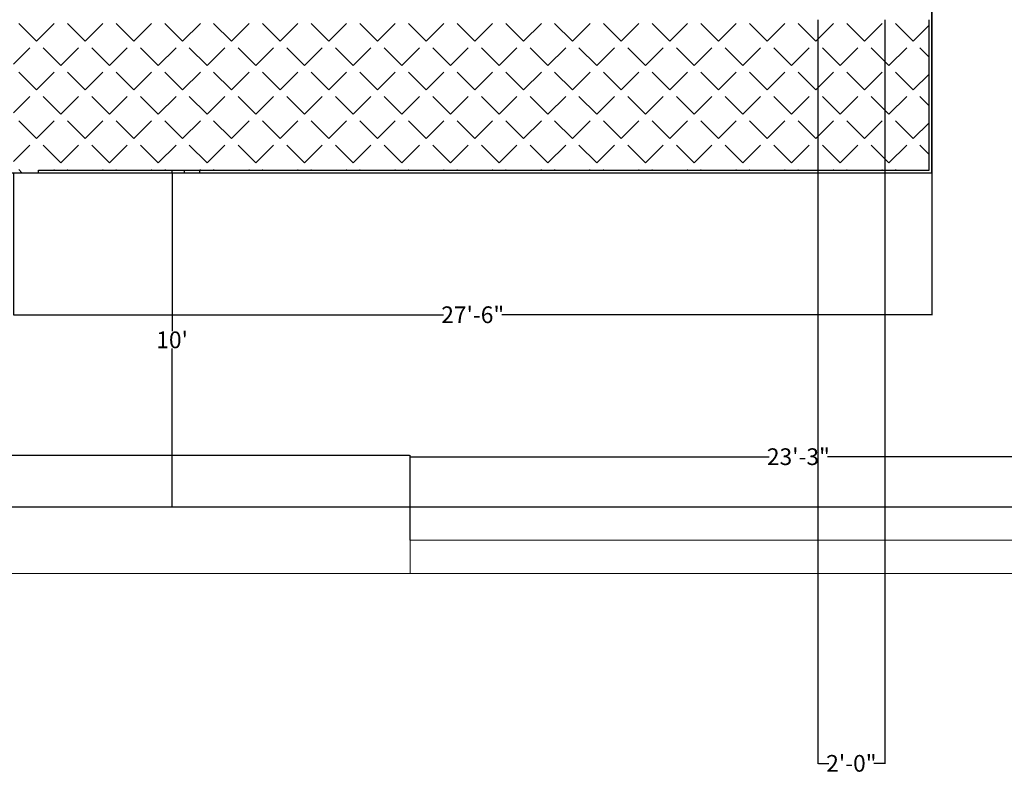
# Model space of a CAD drawing. Units: inches. Extents: x -2181 to 1225, y -80 to 4016.
# Tile 6 of 10: x 668 to 1021, y -80 to 191. Entities that reach past the tile are written whole.
import ezdxf

# ---------------------------------------------------------------- set-up
doc = ezdxf.new("R2010")
doc.units = ezdxf.units.IN
doc.header["$MEASUREMENT"] = 0
for name, color, linetype, lineweight in [('A-ANNO-DIMS', 2, 'Continuous', 18), ('A-FLOR', 7, 'Continuous', 25), ('A-FLOR-PATT', 252, 'Continuous', 13), ('A-WALL', 7, 'Continuous', 35), ('C-PROP', 7, 'Continuous', 30), ('C-ROAD', 8, 'Continuous', 18)]:
    doc.layers.add(name, color=color, linetype=linetype, lineweight=lineweight)
doc.styles.get("Standard").update_dxf_attribs({"font": 'arial.ttf'})
doc.dimstyles.get("Standard").update_dxf_attribs({"dimtxt": 6, "dimasz": 0.18, "dimexe": 0.18, "dimexo": 0.0625, "dimgap": 0.09, "dimtad": 0, "dimtih": 1, "dimtoh": 1, "dimdec": 4, "dimzin": 0, "dimdsep": 46, "dimlunit": 4, "dimtxsty": 'Standard', "dimcen": 0.09, "dimadec": 0, "dimazin": 0, "dimtfac": 1, "dimtdec": 4, "dimtofl": 0, "dimtmove": 0, "dimatfit": 3, "dimfxl": 1, "dimtolj": 1, "dimtzin": 0, "dimarcsym": 0})

# ---------------------------------------------------------------- blocks, each defined once
blk = doc.blocks.new('*D24')
at = {"layer": 'A-ANNO-DIMS', "color": 0, "lineweight": -2, "transparency": 16777216}
for p, q in [((722.51, 136.3), (722.51, 79.64)), ((722.58, 136.48), (722.69, 136.48)), ((722.51, 16.66), (722.51, 73.33)), ((722.58, 16.48), (722.69, 16.48))]:
    blk.add_line(p, q, dxfattribs=at)
at = {"layer": 'A-ANNO-DIMS', "color": 0, "transparency": 16777216}
for points in [[(722.48, 136.3), (722.54, 136.3), (722.51, 136.48)], [(722.48, 16.66), (722.54, 16.66), (722.51, 16.48)]]:
    blk.add_solid(points, dxfattribs=at)
at = {"layer": 'Defpoints', "color": 0, "transparency": 16777216}
for p in [(722.51, 136.48), (722.51, 16.48), (722.51, 16.48)]:
    blk.add_point(p, dxfattribs=at)
at = {"layer": 'A-ANNO-DIMS', "color": 0, "transparency": 16777216, "insert": (722.51, 76.48), "char_height": 6, "attachment_point": 5}
blk.add_mtext("\\A1;10'", dxfattribs=at)
blk = doc.blocks.new('*D60')
at = {"layer": 'A-ANNO-DIMS', "color": 0, "lineweight": -2, "transparency": 16777216}
for p, q in [((665.51, 136.42), (665.51, 85.31)), ((995.51, 136.42), (995.51, 85.31)), ((665.69, 85.49), (820.07, 85.49)), ((995.33, 85.49), (840.96, 85.49))]:
    blk.add_line(p, q, dxfattribs=at)
at = {"layer": 'A-ANNO-DIMS', "color": 0, "transparency": 16777216}
for points in [[(665.69, 85.52), (665.69, 85.46), (665.51, 85.49)], [(995.33, 85.52), (995.33, 85.46), (995.51, 85.49)]]:
    blk.add_solid(points, dxfattribs=at)
at = {"layer": 'Defpoints', "color": 0, "transparency": 16777216}
for p in [(665.51, 136.48), (995.51, 136.48), (995.51, 85.49)]:
    blk.add_point(p, dxfattribs=at)
at = {"layer": 'A-ANNO-DIMS', "color": 0, "transparency": 16777216, "insert": (830.51, 85.49), "char_height": 6, "attachment_point": 5}
blk.add_mtext('\\A1;27\'-6"', dxfattribs=at)
blk = doc.blocks.new('*D68')
at = {"layer": 'A-ANNO-DIMS', "color": 0, "lineweight": -2, "transparency": 16777216}
for p, q in [((331.01, 4.55), (331.01, 35.07)), ((331.19, 34.89), (559.12, 34.89)), ((807.83, 34.89), (579.91, 34.89)), ((808.01, 4.55), (808.01, 35.07))]:
    blk.add_line(p, q, dxfattribs=at)
at = {"layer": 'A-ANNO-DIMS', "color": 0, "transparency": 16777216}
for points in [[(331.19, 34.92), (331.19, 34.86), (331.01, 34.89)], [(807.83, 34.92), (807.83, 34.86), (808.01, 34.89)]]:
    blk.add_solid(points, dxfattribs=at)
at = {"layer": 'Defpoints', "color": 0, "transparency": 16777216}
for p in [(808.01, 34.89), (331.01, 4.48), (808.01, 4.48)]:
    blk.add_point(p, dxfattribs=at)
at = {"layer": 'A-ANNO-DIMS', "color": 0, "transparency": 16777216, "insert": (569.51, 34.89), "char_height": 6, "attachment_point": 5}
blk.add_mtext('\\A1;39\'-9"', dxfattribs=at)
blk = doc.blocks.new('*D69')
at = {"layer": 'A-ANNO-DIMS', "color": 0, "lineweight": -2, "transparency": 16777216}
for p, q in [((808.01, 4.55), (808.01, 34.68)), ((808.19, 34.5), (937.07, 34.5)), ((1086.83, 34.5), (957.96, 34.5)), ((1087.01, 4.55), (1087.01, 34.68))]:
    blk.add_line(p, q, dxfattribs=at)
at = {"layer": 'A-ANNO-DIMS', "color": 0, "transparency": 16777216}
for points in [[(808.19, 34.53), (808.19, 34.47), (808.01, 34.5)], [(1086.83, 34.53), (1086.83, 34.47), (1087.01, 34.5)]]:
    blk.add_solid(points, dxfattribs=at)
at = {"layer": 'Defpoints', "color": 0, "transparency": 16777216}
for p in [(1087.01, 34.5), (808.01, 4.48), (1087.01, 4.48)]:
    blk.add_point(p, dxfattribs=at)
at = {"layer": 'A-ANNO-DIMS', "color": 0, "transparency": 16777216, "insert": (947.51, 34.5), "char_height": 6, "attachment_point": 5}
blk.add_mtext('\\A1;23\'-3"', dxfattribs=at)
blk = doc.blocks.new('*D133')
at = {"layer": 'A-ANNO-DIMS', "color": 0, "lineweight": -2, "transparency": 16777216}
for p, q in [((954.51, 191.42), (954.51, -75.85)), ((978.59, 191.42), (978.59, -75.85)), ((954.69, -75.67), (958.44, -75.67)), ((978.41, -75.67), (974.67, -75.67))]:
    blk.add_line(p, q, dxfattribs=at)
at = {"layer": 'A-ANNO-DIMS', "color": 0, "transparency": 16777216}
for points in [[(954.69, -75.64), (954.69, -75.7), (954.51, -75.67)], [(978.41, -75.64), (978.41, -75.7), (978.59, -75.67)]]:
    blk.add_solid(points, dxfattribs=at)
at = {"layer": 'Defpoints', "color": 0, "transparency": 16777216}
for p in [(954.51, 191.48), (978.59, 191.48), (978.59, -75.67)]:
    blk.add_point(p, dxfattribs=at)
at = {"layer": 'A-ANNO-DIMS', "color": 0, "transparency": 16777216, "insert": (966.55, -75.67), "char_height": 6, "attachment_point": 5}
blk.add_mtext('\\A1;2\'-0"', dxfattribs=at)

msp = doc.modelspace()

# ---------------------------------------------------------------- hatches: boundary and pattern name
at = {"layer": 'A-FLOR-PATT'}
h = msp.add_hatch(dxfattribs=at)
h.set_pattern_fill('ANGLE', color=256, scale=45, angle=45)
h.set_pattern_definition([(45, (0, 0), (-8.75045, 8.75045), [9, -3.375]), (135, (0, 0), (-8.75045, -8.75045), [9, -3.375])])
h.paths.add_polyline_path([(665.51461, 191.48479), (665.51461, 136.48479), (674.51461, 136.48479), (674.51461, 137.48479), (994.51461, 137.48479), (994.51461, 191.48479)])

# ---------------------------------------------------------------- linework, layer by layer
at = {"layer": 'A-FLOR'}
for points in [[(994.51461, 137.48479), (994.51461, 191.48479)], [(98.51461, 136.48479), (995.51461, 136.48479)], [(674.51461, 136.48479), (674.51461, 137.48479)], [(674.51461, 137.48479), (994.51461, 137.48479)], [(722.51461, 136.48479), (722.51461, 137.48479)], [(727.01461, 136.48479), (727.01461, 137.48479)], [(732.51461, 136.48479), (732.51461, 137.48479)]]:
    msp.add_lwpolyline(points, dxfattribs=at)
at = {"layer": 'A-WALL'}
msp.add_lwpolyline([(995.51461, 136.48479), (995.51461, 572.98479), (665.51461, 572.98479)], dxfattribs=at)
at = {"layer": 'C-PROP'}
msp.add_lwpolyline([(7.01461, 16.48479), (1087.01461, 16.48479)], dxfattribs=at)
at = {"layer": 'C-ROAD'}
for q in [(808.01461, -7.51521), (1087.01461, 4.48479)]:
    msp.add_line((808.01461, 4.48479), q, dxfattribs=at)
msp.add_lwpolyline([(7.01461, -7.51521), (1087.01461, -7.51521)], dxfattribs=at)

# ---------------------------------------------------------------- dimensions: what is measured, and where the dimension line sits
at = {"layer": 'A-ANNO-DIMS'}
for base, p1, p2, override, picture, middle in [((978.59298, -75.66522), (954.51171, 191.48478), (978.59298, 191.48478), {"dimdec": 1, "dimlfac": 1, "dimrnd": 0, "dimzin": 1, "dimdsep": 46, "dimlunit": 4, "dimfrac": 2}, '*D133', (966.55234, -75.66522)), ((995.51461, 85.49081), (665.51461, 136.48479), (995.51461, 136.48479), {"dimclrd": 0, "dimclre": 0, "dimclrt": 0}, '*D60', (830.51461, 85.49081)), ((808.01461, 34.89043), (331.01461, 4.48479), (808.01461, 4.48479), {"dimclrd": 0, "dimclre": 0, "dimclrt": 0}, '*D68', (569.51461, 34.89043)), ((1087.01461, 34.50007), (808.01461, 4.48479), (1087.01461, 4.48479), {"dimclrd": 0, "dimclre": 0, "dimclrt": 0}, '*D69', (947.51461, 34.50007))]:
    dim = msp.add_linear_dim(base=base, p1=p1, p2=p2, dimstyle='Standard', override=override, dxfattribs=at)
    dim.commit()
    dim.dimension.update_dxf_attribs({"geometry": picture, "text_midpoint": middle})
dim = msp.add_linear_dim(base=(722.51461, 16.48479), p1=(722.51461, 136.48479), p2=(722.51461, 16.48479), angle=90, dimstyle='Standard', override={"dimclrd": 0, "dimclre": 0, "dimclrt": 0}, dxfattribs=at)
dim.commit()
dim.dimension.update_dxf_attribs({"geometry": '*D24', "text_midpoint": (722.51461, 76.48479)})

doc.saveas('drawing.dxf')
